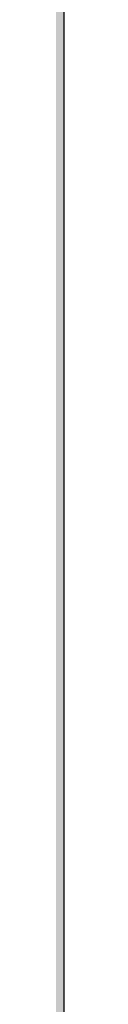
# Model space of a CAD drawing. Units: inches. Extents: x 2091 to 2899, y 967 to 2217.
# Tile 69 of 256: x 2212.144 to 2212.144, y 1101.165 to 1102.499. Entities that reach past the tile are written whole.
import ezdxf

# ---------------------------------------------------------------- set-up
doc = ezdxf.new("R2010")
doc.units = ezdxf.units.IN
doc.layers.add('A-ANNO-DIMS', color=2, linetype='Continuous', lineweight=18)
doc.layers.add('A-WALL-PATT', color=141, linetype='Continuous', lineweight=13, true_color=0xadddf7)
doc.styles.get("Standard").update_dxf_attribs({"font": 'arial.ttf'})
doc.dimstyles.new('ISO-25', dxfattribs={"dimtxt": 4, "dimasz": 4, "dimexe": 1.25, "dimexo": 0.625, "dimtad": 1, "dimdec": 0, "dimlunit": 3, "dimtxsty": 'Standard', "dimcen": 2.5, "dimadec": 0, "dimazin": 0, "dimtfac": 1, "dimtdec": 0, "dimtmove": 0, "dimatfit": 3, "dimfxl": 1, "dimarcsym": 0})

# ---------------------------------------------------------------- blocks, each defined once
blk = doc.blocks.new('*D71')
at = {"layer": 'A-ANNO-DIMS', "color": 0, "lineweight": -2, "transparency": 16777216}
for p, q in [((2212.1436, 1351.2941), (2212.1436, 969.4643)), ((2452.1436, 1351.2941), (2452.1436, 969.4643)), ((2216.1436, 970.7143), (2448.1436, 970.7143))]:
    blk.add_line(p, q, dxfattribs=at)
at = {"layer": 'A-ANNO-DIMS', "color": 0, "transparency": 16777216}
for points in [[(2216.1436, 971.381), (2216.1436, 970.0476), (2212.1436, 970.7143)], [(2448.1436, 971.381), (2448.1436, 970.0476), (2452.1436, 970.7143)]]:
    blk.add_solid(points, dxfattribs=at)
at = {"layer": 'Defpoints', "color": 0, "transparency": 16777216}
for p in [(2212.1436, 1351.9191), (2452.1436, 1351.9191), (2452.1436, 970.7143)]:
    blk.add_point(p, dxfattribs=at)
at = {"layer": 'A-ANNO-DIMS', "color": 0, "transparency": 16777216, "insert": (2332.1436, 973.3816), "char_height": 4, "attachment_point": 5}
blk.add_mtext('20\'-0"', dxfattribs=at)
blk = doc.blocks.new('*D75')
at = {"layer": 'A-ANNO-DIMS', "color": 0, "lineweight": -2, "transparency": 16777216}
for p, q in [((2212.1436, 1274.7941), (2212.1436, 969.4643)), ((2308.1436, 1274.7941), (2308.1436, 969.4643)), ((2216.1436, 970.7143), (2304.1436, 970.7143))]:
    blk.add_line(p, q, dxfattribs=at)
at = {"layer": 'A-ANNO-DIMS', "color": 0, "transparency": 16777216}
for points in [[(2216.1436, 971.381), (2216.1436, 970.0476), (2212.1436, 970.7143)], [(2304.1436, 971.381), (2304.1436, 970.0476), (2308.1436, 970.7143)]]:
    blk.add_solid(points, dxfattribs=at)
at = {"layer": 'Defpoints', "color": 0, "transparency": 16777216}
for p in [(2212.1436, 1275.4191), (2308.1436, 1275.4191), (2308.1436, 970.7143)]:
    blk.add_point(p, dxfattribs=at)
at = {"layer": 'A-ANNO-DIMS', "color": 0, "transparency": 16777216, "insert": (2260.1436, 973.3816), "char_height": 4, "attachment_point": 5}
blk.add_mtext('8\'-0"', dxfattribs=at)
blk = doc.blocks.new('*D91')
at = {"layer": 'A-ANNO-DIMS', "color": 0, "lineweight": -2, "transparency": 16777216}
for p, q in [((2211.6506, 1152.2471), (2098.3113, 1152.2471)), ((2099.5613, 1103.9191), (2099.5613, 1148.2471)), ((2211.5186, 1099.9191), (2098.3113, 1099.9191))]:
    blk.add_line(p, q, dxfattribs=at)
at = {"layer": 'A-ANNO-DIMS', "color": 0, "transparency": 16777216}
for points in [[(2098.8947, 1148.2471), (2100.228, 1148.2471), (2099.5613, 1152.2471)], [(2098.8947, 1103.9191), (2100.228, 1103.9191), (2099.5613, 1099.9191)]]:
    blk.add_solid(points, dxfattribs=at)
at = {"layer": 'Defpoints', "color": 0, "transparency": 16777216}
for p in [(2099.5613, 1152.2471), (2212.2756, 1152.2471), (2212.1436, 1099.9191)]:
    blk.add_point(p, dxfattribs=at)
at = {"layer": 'A-ANNO-DIMS', "color": 0, "transparency": 16777216, "insert": (2096.8681, 1126.0831), "char_height": 4, "attachment_point": 5, "rotation": 90}
blk.add_mtext('4\'-4 1/2"', dxfattribs=at)

msp = doc.modelspace()

# ---------------------------------------------------------------- hatches: boundary and pattern name
at = {"layer": 'A-WALL-PATT'}
h = msp.add_hatch(color=256, dxfattribs=at)
h.dxf.hatch_style = 1
h.paths.add_polyline_path([(2803.1436, 2050.9191), (2203.1436, 2050.9191), (2203.1436, 1090.9191), (2803.1436, 1090.9191)])
h.paths.add_polyline_path([(2635.7989, 1147.5405), (2674.5241, 1147.5405, 0.376086), (2678.5297, 1152.8802), (2678.5297, 1159.5565, 0.333335), (2674.5243, 1163.5618), (2674.5243, 1163.5619), (2674.5243, 1192.9344), (2635.806, 1192.9344), (2597.0876, 1192.9344), (2597.0876, 1163.5618, 0.333335), (2593.0823, 1159.5565), (2593.0823, 1152.8802, 0.376086), (2597.0879, 1147.5405)], flags=0)
h.paths.add_polyline_path([(2436.0104, 1278.2408, 0.000483), (2435.9526, 1278.215, -0.001328), (2435.9356, 1278.1117, -0.001711), (2436.1164, 1278.0408, 0.002185)], flags=0)
h.paths.add_polyline_path([(2794.1436, 1143.4191), (2794.1436, 1347.4191), (2543.3702, 1347.4191), (2543.3702, 1351.9191), (2794.1436, 1351.9191), (2794.1436, 1392.7136), (2793.9474, 1392.7136), (2793.9474, 1473.5369), (2794.1436, 1473.5369), (2794.1436, 1531.9191), (2650.1436, 1531.9191), (2650.1436, 1536.4191), (2794.1436, 1536.4191), (2794.1436, 1692.4191), (2609.3756, 1692.4191), (2609.3756, 1644.4191), (2604.8756, 1644.4191), (2604.8756, 1744.9191), (2609.3756, 1744.9191), (2609.3756, 1696.9191), (2794.1436, 1696.9191), (2794.1436, 1780.9191), (2609.6436, 1780.9191), (2493.8756, 1780.9191), (2493.8756, 1785.4191), (2609.6436, 1785.4191), (2794.1436, 1785.4191), (2794.1436, 1847.9388), (2793.9512, 1847.9388), (2793.9512, 1928.7622), (2794.1436, 1928.7622), (2794.1436, 1941.4191), (2614.1436, 1941.4191), (2614.1436, 1821.4191), (2609.6436, 1821.4191), (2609.6436, 1941.4191), (2392.1436, 1941.4191), (2392.1436, 1819.9191), (2387.6436, 1819.9191), (2387.6436, 1941.4191), (2212.1436, 1941.4191), (2212.1436, 1783.9191), (2392.1436, 1783.9191), (2392.1436, 1780.9191), (2212.1436, 1780.9191), (2212.1436, 1629.4191), (2387.6436, 1629.4191), (2387.6436, 1744.9191), (2392.1436, 1744.9191), (2392.1436, 1627.9191), (2317.1436, 1627.9191), (2317.1436, 1551.4191), (2317.1436, 1536.4191), (2459.3836, 1536.4191), (2459.3836, 1602.3965), (2463.8836, 1602.3965), (2463.8836, 1531.9191), (2456.6436, 1531.9191), (2456.6436, 1529.9191), (2452.1436, 1529.9191), (2452.1436, 1531.9191), (2312.6436, 1531.9191), (2312.6436, 1551.4191), (2306.1436, 1551.4191), (2306.1436, 1555.9191), (2308.1436, 1555.9191), (2308.1436, 1551.4191), (2312.6436, 1551.4191), (2312.6436, 1627.9191), (2212.1436, 1627.9191), (2212.1436, 1555.9191), (2270.1436, 1555.9191), (2270.1436, 1551.4191), (2212.1436, 1551.4191), (2212.1436, 1351.9191), (2272.1436, 1351.9191), (2272.1436, 1347.4191), (2212.1436, 1347.4191), (2212.1436, 1275.4191), (2308.1436, 1275.4191), (2308.1436, 1351.9191), (2452.1436, 1351.9191), (2452.1436, 1493.9191), (2456.6436, 1493.9191), (2456.6436, 1347.4191), (2312.6436, 1347.4191), (2312.6436, 1270.9191), (2212.1436, 1270.9191), (2212.1436, 1099.9191), (2281.2375, 1099.9191), (2282.871, 1110.9138), (2282.0083, 1116.9966), (2278.5577, 1121.4204), (2268.2056, 1128.0562), (2272.0876, 1128.0562), (2273.8129, 1131.927), (2279.4203, 1134.6919), (2285.0278, 1135.2449), (2287.6158, 1137.4568), (2288.0471, 1138.0098), (2289.3411, 1140.7747), (2291.0665, 1139.6687), (2292.3605, 1135.2449), (2295.3798, 1136.9038), (2296.2425, 1135.7979), (2297.1052, 1133.033), (2300.1246, 1138.0098), (2303.1439, 1138.0098), (2304.4379, 1135.7979), (2303.1439, 1133.586), (2306.5946, 1134.6919), (2307.8887, 1133.033), (2310.908, 1135.2449), (2313.9274, 1134.1389), (2315.6269, 1132.4271), (2308.32, 1117.5496), (2290.2038, 1109.8079), (2288.9098, 1103.1721), (2289.2723, 1099.9191), (2434.9182, 1099.9191), (2431.5932, 1124.7881), (2429.9302, 1169.5531), (2430.9272, 1240.5197), (2435.6589, 1238.1861), (2437.1352, 1196.5541), (2438.7982, 1143.9731), (2442.6782, 1111.9981), (2446.5582, 1099.9191), (2794.1436, 1099.9191), (2794.1436, 1138.9191), (2548.0324, 1138.9191), (2548.0324, 1143.4191), (2548.0324, 1148.8191), (2546.6685, 1148.0316), (2528.6857, 1179.1786, 0.256256), (2512.0324, 1148.8191), (2512.0324, 1143.4191), (2512.0324, 1138.9191), (2507.5324, 1138.9191), (2507.5324, 1143.4191), (2507.5324, 1148.8191, 0.256256), (2490.8792, 1179.1786), (2472.8964, 1148.0316), (2471.5324, 1148.8191), (2471.5324, 1143.4191), (2467.0324, 1143.4191), (2467.0324, 1269.9458, 0.039061), (2460.91, 1273.5801), (2467.0324, 1273.5801), (2467.0324, 1286.3254, 0.014511), (2465.2162, 1286.7619), (2467.0324, 1287.0526), (2467.0324, 1323.4191), (2471.5324, 1323.4191), (2471.5324, 1148.8191), (2489.5324, 1179.996), (2490.8964, 1179.2085), (2490.8792, 1179.1786, -0.256256), (2507.5324, 1148.8191), (2507.5324, 1143.4191), (2512.0324, 1143.4191), (2512.0324, 1148.8191, -0.256256), (2528.6857, 1179.1786), (2528.6685, 1179.2085), (2530.0324, 1179.996), (2548.0324, 1148.8191), (2548.0324, 1143.4191)], flags=16)
h.paths.add_polyline_path([(2607.7685, 1200.9451), (2607.7685, 1265.0306), (2597.0876, 1281.052), (2619.7846, 1281.052), (2627.7953, 1337.1269), (2635.7989, 1337.1269), (2643.8167, 1337.1269), (2651.8274, 1281.052), (2674.5243, 1281.052), (2663.8434, 1265.0306), (2663.8434, 1200.9451), (2635.806, 1200.9451)], flags=0)
edge = h.paths.add_edge_path(flags=0)
edge.add_ellipse((13303.8962, 1272.9987), major_axis=(-10595.313, 0), ratio=0.8423038701, start_angle=0.62823722, end_angle=0.6465541, ccw=False)
edge.add_ellipse((2711.7004, 1156.8527), major_axis=(2.2198, 0), ratio=0.842304, start_angle=111.5352, end_angle=180.6282, ccw=False)
edge.add_ellipse((13303.1563, 1272.9987), major_axis=(-10593.0263, 0), ratio=0.8423038695, start_angle=0.52827147, end_angle=0.6465541, ccw=False)
edge.add_line((2710.7646, 1175.3333), (2710.13, 1175.3333))
edge.add_ellipse((2710.13, 1176.5798), major_axis=(1.4798, 0), ratio=0.842304, start_angle=180, end_angle=270, ccw=False)
edge.add_line((2708.6501, 1176.5798), (2708.6501, 1200.7829))
edge.add_ellipse((2710.13, 1200.7829), major_axis=(1.4798, 0), ratio=0.842304, start_angle=90, end_angle=180, ccw=False)
edge.add_line((2710.13, 1202.0294), (2710.4651, 1202.0294))
edge.add_ellipse((13303.1563, 1272.9987), major_axis=(-10593.0263, 0), ratio=0.8423038695, start_angle=-0.09022909, end_angle=0.38386678, ccw=False)
edge.add_ellipse((2710.13, 1290.927), major_axis=(-1.4798, 0), ratio=0.842304, start_angle=0, end_angle=90, ccw=False)
edge.add_line((2708.6501, 1290.927), (2708.6501, 1315.1302))
edge.add_ellipse((2710.13, 1315.1302), major_axis=(-1.4798, 0), ratio=0.842304, start_angle=-90, end_angle=0, ccw=False)
edge.add_line((2710.13, 1316.3767), (2710.7063, 1316.3767))
edge.add_ellipse((3238.4017, 1296.2896), major_axis=(528.234, 0), ratio=0.84230387, start_angle=176.349572, end_angle=177.82005, ccw=False)
edge.add_ellipse((2775.063, 1071.4507), major_axis=(313.3078, 0), ratio=0.84230387, start_angle=102.125966, end_angle=103.780529, ccw=False)
edge.add_ellipse((2775.063, 1078.3057), major_axis=(-305.3029, 0), ratio=0.84230387, start_angle=-79.790461, end_angle=-77.555373, ccw=False)
edge.add_ellipse((2695.1418, 1541.9754), major_axis=(-250.9602, 0), ratio=0.84230387, start_angle=99.256566, end_angle=102.554933)
edge.add_line((2741.4103, 1334.2143), (2747.1325, 1337.3785))
edge.add_ellipse((2747.5386, 1336.8575), major_axis=(-0.7399, 0), ratio=0.842304, start_angle=270, end_angle=307.9331, ccw=False)
edge.add_ellipse((2747.5386, 1336.8575), major_axis=(-0.7399, 0), ratio=0.842304, start_angle=232.0669, end_angle=270, ccw=False)
edge.add_line((2747.9447, 1337.3785), (2753.6669, 1334.2143))
edge.add_ellipse((2799.9355, 1541.9754), major_axis=(250.9602, 0), ratio=0.84230387, start_angle=257.445067, end_angle=260.743434)
edge.add_ellipse((2720.0142, 1078.3057), major_axis=(305.3029, 0), ratio=0.84230387, start_angle=77.555373, end_angle=79.790461, ccw=False)
edge.add_ellipse((2720.0142, 1071.4507), major_axis=(-313.3078, 0), ratio=0.84230387, start_angle=256.219471, end_angle=257.874034, ccw=False)
edge.add_ellipse((2256.6755, 1296.2896), major_axis=(-528.234, 0), ratio=0.84230387, start_angle=182.17995, end_angle=183.650428, ccw=False)
edge.add_line((2784.3709, 1316.3767), (2784.9472, 1316.3767))
edge.add_ellipse((2784.9472, 1315.1302), major_axis=(1.4798, 0), ratio=0.842304, start_angle=0, end_angle=90, ccw=False)
edge.add_line((2786.4271, 1315.1302), (2786.4271, 1290.927))
edge.add_ellipse((2784.9472, 1290.927), major_axis=(1.4798, 0), ratio=0.842304, start_angle=270, end_angle=360, ccw=False)
edge.add_ellipse((-7808.0791, 1272.9987), major_axis=(10593.0263, 0), ratio=0.8423038695, start_angle=-0.38386678, end_angle=0.09022909, ccw=False)
edge.add_line((2784.6122, 1202.0294), (2784.9472, 1202.0294))
edge.add_ellipse((2784.9472, 1200.7829), major_axis=(1.4798, 0), ratio=0.842304, start_angle=0, end_angle=90, ccw=False)
edge.add_line((2786.4271, 1200.7829), (2786.4271, 1176.5798))
edge.add_ellipse((2784.9472, 1176.5798), major_axis=(-1.4798, 0), ratio=0.842304, start_angle=90, end_angle=180, ccw=False)
edge.add_line((2784.9472, 1175.3333), (2784.3126, 1175.3333))
edge.add_ellipse((-7808.0791, 1272.9987), major_axis=(10593.0263, 0), ratio=0.8423038695, start_angle=-0.6186432, end_angle=-0.52827147, ccw=False)
edge.add_ellipse((2783.3768, 1156.8527), major_axis=(-2.2198, 0), ratio=0.842304, start_angle=179.3718, end_angle=248.4648, ccw=False)
edge.add_ellipse((-7808.819, 1272.9987), major_axis=(-10595.313, 0), ratio=0.8423038658, start_angle=179.35344592, end_angle=179.3717628, ccw=False)
edge.add_ellipse((2780.2973, 1153.5008), major_axis=(-5.2464, 0), ratio=0.842304, start_angle=90, end_angle=179.3534, ccw=False)
edge.add_line((2780.2973, 1149.0817), (2714.7799, 1149.0817))
edge.add_ellipse((2714.7799, 1153.5008), major_axis=(5.2464, 0), ratio=0.842304, start_angle=180.6466, end_angle=270, ccw=False)
edge = h.paths.add_edge_path(flags=0)
edge.add_line((2718.1874, 1151.0078), (2718.1874, 1170.4724))
edge.add_ellipse((2721.1471, 1170.4724), major_axis=(-2.9597, 0), ratio=0.842304, start_angle=-90, end_angle=0, ccw=False)
edge.add_line((2721.1471, 1172.9653), (2773.9302, 1172.9653))
edge.add_ellipse((2773.9302, 1170.4724), major_axis=(-2.9597, 0), ratio=0.842304, start_angle=180, end_angle=270, ccw=False)
edge.add_line((2776.8899, 1170.4724), (2776.8899, 1151.0078))
edge.add_line((2776.8899, 1151.0078), (2718.1874, 1151.0078))
edge = h.paths.add_edge_path(flags=0)
edge.add_line((2718.1874, 1180.2342), (2718.1874, 1199.0578))
edge.add_ellipse((2747.5386, 1320.3986), major_axis=(147.0179, 0), ratio=0.84230387, start_angle=256.401865, end_angle=283.598135)
edge.add_line((2776.8899, 1199.0578), (2776.8899, 1180.2342))
edge.add_ellipse((2747.5386, 1301.575), major_axis=(147.0179, 0), ratio=0.84230387, start_angle=256.401865, end_angle=283.598135, ccw=False)
edge = h.paths.add_edge_path(flags=0)
edge.add_ellipse((13303.1563, 1272.9987), major_axis=(-10591.5465, 0), ratio=0.8423038696, start_angle=0.05559431, end_angle=0.37776419, ccw=False)
edge.add_line((2711.6169, 1262.7217), (2715.6674, 1249.4954))
edge.add_ellipse((6413.892, 1241.6919), major_axis=(-3698.2362, 0), ratio=0.84230387, start_angle=-0.1208974, end_angle=0.3640763)
edge.add_line((2715.761, 1218.1925), (2711.9343, 1203.1674))
edge = h.paths.add_edge_path(flags=0)
edge.add_line((2718.1874, 1251.0746), (2716.0025, 1267.4504))
edge.add_ellipse((2742.1512, 1202.1895), major_axis=(81.7726, 0), ratio=0.8423039, start_angle=94.277421, end_angle=111.834954, ccw=False)
edge.add_line((2737.0097, 1270.9306), (2758.0675, 1270.9306))
edge.add_ellipse((2752.9261, 1202.1895), major_axis=(81.7726, 0), ratio=0.8423039, start_angle=68.165046, end_angle=85.722579, ccw=False)
edge.add_line((2779.0747, 1267.4504), (2776.8899, 1251.0746))
edge.add_ellipse((2750.3381, 1187.8854), major_axis=(79.5797, 0), ratio=0.8423039, start_angle=67.208085, end_angle=85.12993)
edge.add_line((2756.0347, 1254.7437), (2739.0426, 1254.7437))
edge.add_ellipse((2744.7392, 1187.8854), major_axis=(79.5797, 0), ratio=0.8423039, start_angle=94.87007, end_angle=112.791915)
edge = h.paths.add_edge_path(flags=0)
edge.add_line((2783.1429, 1203.1674), (2779.3162, 1218.1925))
edge.add_ellipse((-918.8147, 1241.6919), major_axis=(3698.2362, 0), ratio=0.84230387, start_angle=-0.3640763, end_angle=0.1208974)
edge.add_line((2779.4098, 1249.4954), (2783.4604, 1262.7217))
edge.add_ellipse((-7808.0791, 1272.9987), major_axis=(-10591.5465, 0), ratio=0.8423038695, start_angle=179.62223581, end_angle=179.94440569, ccw=False)
edge = h.paths.add_edge_path(flags=0)
edge.add_ellipse((2734.2009, 1286.6904), major_axis=(-0.3566, 6.3401), ratio=0.603834, start_angle=89.00201, end_angle=253.65741, ccw=False)
edge.add_line((2730.369, 1286.5418), (2730.369, 1301.352))
edge.add_line((2730.369, 1301.352), (2735.9133, 1305.2148))
edge.add_ellipse((2736.3849, 1304.7346), major_axis=(0.7399, 0), ratio=0.842304, start_angle=90, end_angle=134.4802, ccw=False)
edge.add_line((2736.3849, 1305.3578), (2738.0328, 1305.3578))
edge.add_line((2738.0328, 1305.3578), (2738.0328, 1307.7079))
edge.add_ellipse((2794.2016, 1307.7079), major_axis=(56.1689, 0), ratio=0.8423039, start_angle=150.56143, end_angle=180, ccw=False)
edge.add_ellipse((2700.8756, 1307.7079), major_axis=(-56.1689, 0), ratio=0.8423039, start_angle=180, end_angle=209.43857, ccw=False)
edge.add_line((2757.0444, 1307.7079), (2757.0444, 1305.3578))
edge.add_line((2757.0444, 1305.3578), (2758.6923, 1305.3578))
edge.add_ellipse((2758.6923, 1304.7346), major_axis=(-0.7399, 0), ratio=0.842304, start_angle=225.5198, end_angle=270, ccw=False)
edge.add_line((2759.1639, 1305.2148), (2764.7082, 1301.352))
edge.add_line((2764.7082, 1301.352), (2764.7082, 1286.5418))
edge.add_ellipse((2760.8763, 1286.6904), major_axis=(0.3566, 6.3401), ratio=0.603834, start_angle=106.34259, end_angle=270.99799, ccw=False)
edge.add_line((2757.0444, 1285.7971), (2757.0444, 1307.7079))
edge.add_ellipse((2700.8756, 1307.7079), major_axis=(-56.1689, 0), ratio=0.8423039, start_angle=180, end_angle=209.43857)
edge.add_ellipse((2794.2016, 1307.7079), major_axis=(56.1689, 0), ratio=0.8423039, start_angle=150.56143, end_angle=180)
edge.add_line((2738.0328, 1307.7079), (2738.0328, 1285.7971))
h.paths.add_polyline_path([(2417.8123, 1104.4497), (2413.4923, 1102.5297), (2410.6123, 1103.9697), (2409.1723, 1106.3697), (2407.2523, 1107.3297), (2406.2923, 1109.7297), (2405.3323, 1114.0497), (2405.3323, 1117.8897), (2406.2923, 1120.1297), (2407.2523, 1119.8097), (2408.8483, 1118.3277), (2410.1739, 1119.4242), (2410.2113, 1120.4057), (2411.0407, 1121.4191), (2410.6993, 1119.8587), (2410.1739, 1119.4242), (2410.0885, 1117.1761), (2411.1328, 1116.2063), (2413.9723, 1119.3297), (2416.8523, 1120.7697), (2416.8697, 1120.7988), (2417.0351, 1119.4051), (2417.8962, 1118.1434), (2418.2923, 1118.3697), (2419.5444, 1120.0393), (2419.3609, 1118.3875), (2419.0321, 1119.3562), (2418.3989, 1118.5119), (2419.2523, 1114.5297), (2418.7941, 1107.1988)], flags=0)
h.paths.add_polyline_path([(2508.8702, 1347.4191), (2508.3702, 1347.4191), (2508.3702, 1351.9191), (2508.8702, 1351.9191)], flags=0)
h.paths.add_polyline_path([(2473.3702, 1347.4191), (2472.3702, 1347.4191), (2467.8702, 1347.4191), (2467.8702, 1455.4191), (2472.3702, 1455.4191), (2472.3702, 1352.4191), (2473.3702, 1352.4191)], flags=0)
h.paths.add_polyline_path([(2352.1062, 1217.4462), (2349.2262, 1218.8862), (2347.7862, 1221.2862), (2345.8662, 1222.2462), (2344.9062, 1224.6462), (2343.9462, 1228.9662), (2343.9462, 1232.8062), (2344.9062, 1235.0462), (2345.8662, 1234.7262), (2347.4623, 1233.2442), (2348.7879, 1234.3407), (2348.8252, 1235.3222), (2349.6547, 1236.3355), (2349.3132, 1234.7752), (2348.7879, 1234.3407), (2348.7024, 1232.0926), (2349.7468, 1231.1228), (2352.5862, 1234.2462), (2355.4662, 1235.6862), (2355.4837, 1235.7153), (2355.649, 1234.3216), (2356.5102, 1233.0599), (2356.9062, 1233.2862), (2358.1584, 1234.9558), (2357.9749, 1233.304), (2357.6461, 1234.2726), (2357.0129, 1233.4284), (2357.8662, 1229.4462), (2357.4081, 1222.1153), (2356.4262, 1219.3662)], flags=0)
h.paths.add_polyline_path([(2348.2968, 1112.2244), (2347.0138, 1112.3104), (2345.5298, 1114.1274), (2345.7318, 1115.8584), (2346.8118, 1116.9824), (2346.8118, 1114.6464), (2345.8668, 1114.2144), (2346.8798, 1114.3004)], flags=0)
h.paths.add_polyline_path([(2347.0138, 1110.9264), (2346.2718, 1110.4934), (2346.6098, 1111.1864)], flags=0)
h.paths.add_polyline_path([(2345.8668, 1118.1944), (2345.5298, 1117.3294), (2343.7078, 1118.0214), (2344.3828, 1118.6264)], flags=0)
h.paths.add_polyline_path([(2346.6768, 1109.2824), (2346.0698, 1108.0714), (2345.8668, 1110.0614)], flags=0)
h.paths.add_polyline_path([(2345.0568, 1119.7514), (2343.6398, 1119.7514), (2343.9778, 1121.1354)], flags=0)
h.paths.add_polyline_path([(2345.2598, 1116.5504), (2345.1248, 1115.8584), (2344.9218, 1115.6854), (2344.7198, 1116.3774)], flags=0)
h.paths.add_polyline_path([(2345.6648, 1112.3104), (2345.4618, 1111.5324), (2344.0448, 1111.9644), (2344.6518, 1112.5704)], flags=0)
h.paths.add_polyline_path([(2345.1918, 1113.3494), (2344.4498, 1113.8684), (2344.7198, 1114.3874)], flags=0)
h.paths.add_polyline_path([(2344.6518, 1116.8094), (2344.1798, 1115.6854), (2344.6518, 1115.3394), (2343.9098, 1114.9064), (2343.0328, 1115.9444), (2343.6398, 1116.4634)], flags=0)
h.paths.add_polyline_path([(2345.8668, 1106.6864), (2344.9898, 1105.5624), (2344.5168, 1106.6004)], flags=0)
h.paths.add_polyline_path([(2344.8548, 1110.0614), (2344.5168, 1109.2824), (2344.1128, 1109.7154)], flags=0)
h.paths.add_polyline_path([(2344.0448, 1113.5224), (2343.4378, 1113.0894), (2342.7628, 1113.9544)], flags=0)
h.paths.add_polyline_path([(2344.3148, 1111.0124), (2342.9648, 1110.3204), (2342.9648, 1111.0994)], flags=0)
h.paths.add_polyline_path([(2345.1248, 1104.6974), (2344.5848, 1103.7454), (2344.4498, 1104.2644)], flags=0)
h.paths.add_polyline_path([(2342.8298, 1121.2224), (2341.7498, 1120.5304), (2340.5358, 1121.0494), (2340.1308, 1121.8284), (2340.6708, 1122.9524), (2341.1428, 1121.8284), (2341.6148, 1122.0014)], flags=0)
h.paths.add_polyline_path([(2342.9648, 1119.7514), (2343.0328, 1118.4534), (2342.0878, 1118.0214), (2342.0198, 1119.4914)], flags=0)
h.paths.add_polyline_path([(2342.6948, 1116.8964), (2341.9528, 1116.6364), (2342.0198, 1117.3294)], flags=0)
h.paths.add_polyline_path([(2343.0328, 1112.2244), (2342.0198, 1111.7914), (2341.5478, 1112.2244), (2342.3578, 1113.3494)], flags=0)
h.paths.add_polyline_path([(2343.7748, 1104.4374), (2342.6278, 1102.8804), (2342.6948, 1104.6104), (2343.4378, 1105.1294)], flags=0)
h.paths.add_polyline_path([(2342.0198, 1115.0794), (2340.8058, 1115.5124), (2340.9408, 1116.3774)], flags=0)
h.paths.add_polyline_path([(2341.4808, 1120.0974), (2341.4808, 1119.4054), (2341.0758, 1119.5784), (2341.1428, 1120.0974)], flags=0)
h.paths.add_polyline_path([(2341.8178, 1114.4734), (2340.9408, 1113.0894), (2340.8058, 1114.5604)], flags=0)
h.paths.add_polyline_path([(2341.1428, 1118.5404), (2340.9408, 1116.9824), (2339.0508, 1117.6754), (2339.0508, 1118.6264)], flags=0)
h.paths.add_polyline_path([(2342.6948, 1101.6684), (2341.9528, 1101.8414), (2342.5598, 1102.3614)], flags=0)
h.paths.add_polyline_path([(2340.3328, 1119.6654), (2338.4438, 1119.5784), (2337.9038, 1120.3574), (2339.6578, 1120.6164)], flags=0)
h.paths.add_polyline_path([(2340.3328, 1115.3394), (2340.0628, 1113.6954), (2339.3878, 1115.3394)], flags=0)
h.paths.add_polyline_path([(2341.8178, 1103.8314), (2341.5478, 1102.8804), (2341.1428, 1103.6584)], flags=0)
h.paths.add_polyline_path([(2339.0508, 1122.8664), (2337.2958, 1121.8284), (2337.0938, 1123.1254), (2337.7688, 1123.8184)], flags=0)
h.paths.add_polyline_path([(2339.1178, 1121.7414), (2338.8478, 1121.2224), (2338.1738, 1121.0494), (2338.3758, 1121.5684)], flags=0)
h.paths.add_polyline_path([(2339.1858, 1119.3194), (2338.6458, 1118.7134), (2338.2408, 1118.1074), (2338.2408, 1118.8864)], flags=0)
h.paths.add_polyline_path([(2341.1428, 1101.9284), (2340.6028, 1101.2364), (2340.0628, 1101.8414), (2340.6028, 1102.3614)], flags=0)
h.paths.add_polyline_path([(2337.6338, 1117.7614), (2336.6208, 1118.2804), (2337.2958, 1118.9724)], flags=0)
h.paths.add_polyline_path([(2336.8238, 1119.5784), (2334.7988, 1118.9724), (2335.2038, 1120.3574), (2336.5538, 1120.8764)], flags=0)
h.paths.add_polyline_path([(2339.1178, 1100.4574), (2337.3638, 1100.5434), (2336.7558, 1101.2364)], flags=0)
h.paths.add_polyline_path([(2336.3508, 1122.4334), (2336.0138, 1121.9144), (2334.9338, 1122.4334), (2334.5288, 1123.4714), (2335.7438, 1122.7794)], flags=0)
h.paths.add_polyline_path([(2334.7318, 1120.8764), (2334.2588, 1120.3574), (2334.0568, 1120.7894), (2334.5968, 1121.3084)], flags=0)
h.paths.add_polyline_path([(2334.4618, 1122.1744), (2332.5718, 1121.3084), (2331.3568, 1122.1744), (2332.0998, 1122.8664)], flags=0)
h.paths.add_polyline_path([(2334.2588, 1118.5404), (2333.3818, 1118.4534), (2333.6518, 1119.3194)], flags=0)
h.paths.add_polyline_path([(2335.5418, 1102.2744), (2334.1918, 1102.6204), (2335.2718, 1103.3124)], flags=0)
h.paths.add_polyline_path([(2332.7068, 1119.6654), (2331.6948, 1120.4434), (2332.5048, 1120.7894)], flags=0)
h.paths.add_polyline_path([(2334.7318, 1101.1494), (2333.5168, 1101.5824), (2333.9888, 1101.7554)], flags=0)
h.paths.add_polyline_path([(2332.6398, 1116.6364), (2331.0868, 1116.2904), (2331.9648, 1118.1944)], flags=0)
h.paths.add_polyline_path([(2330.7498, 1121.5684), (2330.2768, 1120.2704), (2328.5228, 1119.3194), (2328.9948, 1121.0494)], flags=0)
h.paths.add_polyline_path([(2330.7498, 1118.6264), (2330.0078, 1117.5024), (2329.8728, 1118.0214)], flags=0)
h.paths.add_polyline_path([(2332.0998, 1102.3614), (2330.5468, 1102.0144), (2331.6948, 1102.9664)], flags=0)
h.paths.add_polyline_path([(2329.5348, 1113.6084), (2329.0628, 1112.3104), (2328.5898, 1113.3494)], flags=0)
h.paths.add_polyline_path([(2328.3878, 1117.8484), (2327.5098, 1116.5504), (2327.1728, 1117.7614)], flags=0)
h.paths.add_polyline_path([(2329.7378, 1106.5134), (2329.5348, 1105.3024), (2328.2528, 1106.0814)], flags=0)
h.paths.add_polyline_path([(2328.6578, 1114.3874), (2328.0498, 1114.1274), (2328.3198, 1114.9064)], flags=0)
h.paths.add_polyline_path([(2328.3198, 1112.2244), (2327.1058, 1112.1374), (2326.7008, 1112.6564)], flags=0)
h.paths.add_polyline_path([(2326.9028, 1115.2524), (2326.7008, 1114.1274), (2325.2158, 1113.6084), (2326.0928, 1115.3394)], flags=0)
h.paths.add_polyline_path([(2326.6328, 1108.3304), (2326.0928, 1107.3794), (2325.8908, 1108.5034), (2326.4978, 1109.1094)], flags=0)
h.paths.add_polyline_path([(2615.1436, 1531.9191), (2609.6436, 1531.9191), (2609.6436, 1620.4191), (2614.1436, 1620.4191), (2614.1436, 1536.4191), (2615.1436, 1536.4191)], flags=0)
h.paths.add_polyline_path([(2545.1436, 1563.4191), (2464.1436, 1563.4191), (2464.1436, 1632.4191), (2509.1436, 1632.4191), (2509.1436, 1627.9191), (2509.1436, 1603.9191), (2468.6436, 1603.9191), (2468.6436, 1567.9191), (2540.6436, 1567.9191), (2540.6436, 1591.9191), (2545.1436, 1591.9191)], flags=0)
h.paths.add_polyline_path([(2388.969, 1549.9857), (2357.4342, 1549.9857), (2357.4342, 1623.3608), (2399.3628, 1623.3608), (2435.6895, 1623.3608), (2435.5925, 1602.5593), (2435.5925, 1602.3965), (2388.969, 1602.3965)], flags=0)
h.paths.add_polyline_path([(2388.8806, 1555.8092), (2374.9044, 1555.8092), (2374.9044, 1600.5716), (2374.9044, 1615.4576), (2406.3509, 1615.4576), (2406.3509, 1618.9394), (2412.1743, 1615.4576), (2406.3509, 1611.9759), (2406.3509, 1615.4576), (2388.8806, 1615.4576)], flags=0)
h.paths.add_polyline_path([(2568.8756, 1644.4191), (2453.3756, 1644.4191), (2453.3756, 1785.4191), (2457.8756, 1785.4191), (2457.8756, 1648.9191), (2568.8756, 1648.9191)], flags=0)
h.paths.add_polyline_path([(2212.1436, 1945.9191), (2212.1436, 2041.9191), (2794.1436, 2041.9191), (2794.1436, 1945.9191)], flags=16)
h.paths.add_polyline_path([(2271.0827, 1964.3172), (2776.853, 1964.3172), (2776.853, 2037.1696), (2271.0827, 2037.1696)], flags=8)
h.paths.add_polyline_path([(2380.6493, 1536.8241), (2461.0408, 1536.8241), (2461.0408, 1554.6526), (2380.6493, 1554.6526)], flags=8)
h.paths.add_polyline_path([(2240.7557, 1609.7255), (2309.1858, 1609.7255), (2309.1858, 1617.6982), (2240.7557, 1617.6982)], flags=8)
h.paths.add_polyline_path([(2212.6773, 1313.5041), (2282.5915, 1313.5041), (2282.5915, 1322.7452), (2212.6773, 1322.7452)], flags=8)
h.paths.add_polyline_path([(2457.112, 1114.7786), (2558.4816, 1114.7786), (2558.4816, 1142.2197), (2457.112, 1142.2197)], flags=8)
h.paths.add_polyline_path([(2473.4423, 1273.0101), (2604.6412, 1273.0101), (2604.6412, 1318.3469), (2473.4423, 1318.3469)], flags=8)
h.paths.add_polyline_path([(2638.8763, 1626.9774), (2684.2504, 1627.9767), (2684.0385, 1637.5975), (2638.6644, 1636.5982)], flags=8)
h.paths.add_polyline_path([(2537.5906, 1453.7934), (2628.3895, 1453.7934), (2628.3895, 1475.3448), (2537.5906, 1475.3448)], flags=8)
h.paths.add_polyline_path([(2504.1376, 1714.6324), (2554.6472, 1714.6324), (2554.6472, 1730.2377), (2504.1376, 1730.2377)], flags=8)
h.paths.add_polyline_path([(2487.5012, 1575.6519), (2535.0971, 1575.6519), (2535.0971, 1598.3776), (2487.5012, 1598.3776)], flags=8)
h.paths.add_polyline_path([(2709.0994, 1735.7103), (2740.0166, 1735.7103), (2740.0166, 1749.9376), (2709.0994, 1749.9376)], flags=8)
h.paths.add_polyline_path([(2442.4384, 1792.1717), (2564.7288, 1792.1717), (2564.7288, 1842.0002), (2442.4384, 1842.0002)], flags=8)
h.paths.add_polyline_path([(2655.8158, 1809.6441), (2789.5201, 1806.6938), (2790.085, 1832.2916), (2656.3806, 1835.2419)], flags=8)
h.paths.add_polyline_path([(2234.8427, 1797.7201), (2368.5929, 1794.7689), (2369.1607, 1820.5041), (2235.4106, 1823.4554)], flags=8)
h.paths.add_polyline_path([(2245.1385, 1644.0063), (2398.4277, 1640.6239), (2398.9948, 1666.3248), (2245.7056, 1669.7073)], flags=8)
h.paths.add_polyline_path([(2306.1428, 1431.1685), (2413.7683, 1428.7937), (2414.3331, 1454.3915), (2306.7077, 1456.7664)], flags=8)
h.paths.add_polyline_path([(2306.8346, 1458.2331), (2393.3805, 1456.3234), (2393.9328, 1481.3544), (2307.3869, 1483.2641)], flags=8)

# ---------------------------------------------------------------- dimensions: what is measured, and where the dimension line sits
at = {"layer": 'A-ANNO-DIMS'}
for base, p1, p2, picture, middle in [((2452.1436, 970.7143), (2212.1436, 1351.9191), (2452.1436, 1351.9191), '*D71', (2332.1436, 973.3816)), ((2308.1436, 970.7143), (2212.1436, 1275.4191), (2308.1436, 1275.4191), '*D75', (2260.1436, 973.3816))]:
    dim = msp.add_linear_dim(base=base, p1=p1, p2=p2, dimstyle='ISO-25', override={"dimdec": 1, "dimlfac": 1, "dimrnd": 0, "dimzin": 1, "dimdsep": 46, "dimlunit": 4, "dimfrac": 2}, dxfattribs=at)
    dim.commit()
    dim.dimension.update_dxf_attribs({"geometry": picture, "text_midpoint": middle})
dim = msp.add_linear_dim(base=(2099.5613, 1152.2471), p1=(2212.1436, 1099.9191), p2=(2212.2756, 1152.2471), angle=90, dimstyle='ISO-25', override={"dimdec": 1, "dimlfac": 1, "dimrnd": 0, "dimzin": 1, "dimdsep": 46, "dimlunit": 4, "dimfrac": 2}, dxfattribs=at)
dim.commit()
dim.dimension.update_dxf_attribs({"geometry": '*D91', "text_midpoint": (2096.8681, 1126.0831)})

doc.saveas('drawing.dxf')
